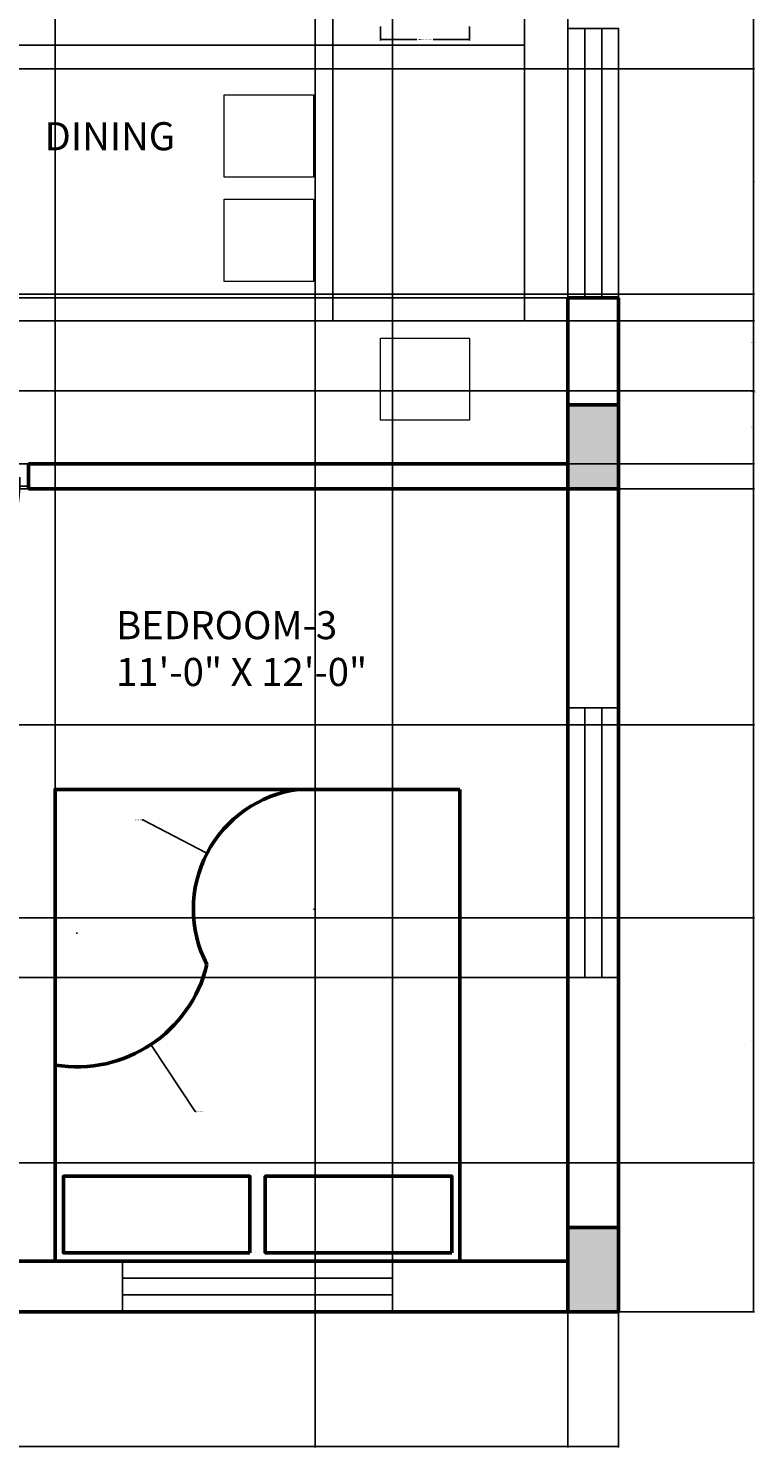
# Model space of a CAD drawing. Units: inches. Extents: x 2480 to 2840, y 795 to 1323.
# Tile 2 of 4: x 2711 to 2840, y 795 to 1047. Entities that reach past the tile are written whole.
import ezdxf

# ---------------------------------------------------------------- set-up
doc = ezdxf.new("R2010")
doc.units = ezdxf.units.IN
for name, color, linetype, lineweight in [('A-ANNO-DIMS', 2, 'Continuous', 18), ('A-AREA-IDEN', 7, 'Continuous', 25), ('COLUMN', 240, 'Continuous', 50), ('door', 140, 'Continuous', 25), ('Furniture', 9, 'Continuous', 18), ('wall', 7, 'Continuous', 50), ('window', 201, 'Continuous', 25)]:
    doc.layers.add(name, color=color, linetype=linetype, lineweight=lineweight)
doc.styles.get("Standard").update_dxf_attribs({"font": 'arial.ttf'})
doc.dimstyles.get("Standard").update_dxf_attribs({"dimtxt": 0.18, "dimasz": 0.18, "dimexe": 0.18, "dimexo": 0.0625, "dimgap": 0.09, "dimtad": 0, "dimtih": 1, "dimtoh": 1, "dimdec": 4, "dimzin": 0, "dimdsep": 46, "dimtxsty": 'Standard', "dimcen": 0.09, "dimadec": 0, "dimazin": 0, "dimtfac": 1, "dimtdec": 4, "dimtofl": 0, "dimtmove": 0, "dimatfit": 3, "dimfxl": 1, "dimtolj": 1, "dimtzin": 0, "dimarcsym": 0})

# ---------------------------------------------------------------- blocks, each defined once
blk = doc.blocks.new('w1')
at = {"layer": 'window'}
for p, q in [((2922.2, 1100.57), (2922.2, 1052.57)), ((2925.2, 1100.57), (2925.2, 1052.57))]:
    blk.add_line(p, q, dxfattribs=at)
blk.add_lwpolyline([(2919.2, 1052.57), (2928.2, 1052.57), (2928.2, 1100.57), (2919.2, 1100.57)], close=True, dxfattribs=at)
blk = doc.blocks.new('d1')
at = {"layer": 'door'}
blk.add_line((3049.73, 1052.02), (3085.73, 1052.02), dxfattribs=at)
blk.add_lwpolyline([(3051.23, 1054.52), (3052.73, 1054.52), (3052.73, 1087.52), (3051.23, 1087.52)], close=True, dxfattribs=at)
for points in [[(3052.73, 1052.02), (3049.73, 1052.02), (3049.73, 1056.02), (3051.23, 1056.02), (3051.23, 1054.52), (3052.73, 1054.52), (3052.73, 1052.02)], [(3082.73, 1052.02), (3085.73, 1052.02), (3085.73, 1056.02), (3084.23, 1056.02), (3084.23, 1054.52), (3082.73, 1054.52), (3082.73, 1052.02)]]:
    blk.add_lwpolyline(points, dxfattribs=at)
blk.add_arc((3051.23, 1054.52), 33.03, 2.6026, 87.3974, dxfattribs=at)
blk = doc.blocks.new('BED')
at = {"layer": 'wall'}
for points in [[(3037.98, 1220.47), (3109.98, 1220.47), (3109.98, 1304.47), (3037.98, 1304.47)], [(3039.4, 1302.95), (3072.6, 1302.95), (3072.6, 1289.33), (3039.4, 1289.33)], [(3075.32, 1302.95), (3108.52, 1302.95), (3108.52, 1289.33), (3075.32, 1289.33)]]:
    blk.add_lwpolyline(points, close=True, dxfattribs=at)
for centre, radius, start, end in [((3106.11, 1246.04), 23.81, 80.6483, 166.366), ((3063.91, 1241.76), 21.48, 277.4854, 27.4236)]:
    blk.add_arc(centre, radius, start, end, dxfattribs=at)
blk = doc.blocks.new('C')
at = {"layer": 'COLUMN'}
h = blk.add_hatch(color=256, dxfattribs=at)
h.dxf.hatch_style = 1
h.paths.add_polyline_path([(3016.24, 1218.72), (3031.24, 1218.72), (3031.24, 1227.72), (3016.24, 1227.72)])
blk.add_lwpolyline([(3016.24, 1218.72), (3031.24, 1218.72), (3031.24, 1227.72), (3016.24, 1227.72)], close=True, dxfattribs=at)
blk = doc.blocks.new('CHAIR-DINING')
blk.add_lwpolyline([(15.88, 0), (0, 0), (0, 14.61), (15.88, 14.61)], close=True)
blk = doc.blocks.new('*D26')
at = {"layer": 'A-ANNO-DIMS', "color": 0, "lineweight": -2, "transparency": 16777216}
for p, q in [((2773.57, 1047.6), (2773.57, 1045.1)), ((2789.45, 1047.6), (2789.45, 1045.1)), ((2773.75, 1045.28), (2780.09, 1045.28)), ((2789.27, 1045.28), (2782.94, 1045.28))]:
    blk.add_line(p, q, dxfattribs=at)
at = {"layer": 'A-ANNO-DIMS', "color": 0, "transparency": 16777216}
for points in [[(2773.75, 1045.31), (2773.75, 1045.25), (2773.57, 1045.28)], [(2789.27, 1045.31), (2789.27, 1045.25), (2789.45, 1045.28)]]:
    blk.add_solid(points, dxfattribs=at)
at = {"layer": 'Defpoints', "color": 0, "transparency": 16777216}
for p in [(2773.57, 1047.66), (2789.45, 1047.66), (2789.45, 1045.28)]:
    blk.add_point(p, dxfattribs=at)
at = {"layer": 'A-ANNO-DIMS', "color": 0, "transparency": 16777216, "insert": (2781.51, 1045.28), "char_height": 0.18, "attachment_point": 5}
blk.add_mtext('\\A1;DINING CHAIR 16 TYP.', dxfattribs=at)
blk = doc.blocks.new('*D28')
at = {"layer": 'A-ANNO-DIMS', "color": 0, "lineweight": -2, "transparency": 16777216}
for p, q in [((2503.95, 836.18), (2503.95, 794.56)), ((2815.95, 818.68), (2815.95, 794.56)), ((2504.13, 794.74), (2659.67, 794.74)), ((2815.77, 794.74), (2660.24, 794.74))]:
    blk.add_line(p, q, dxfattribs=at)
at = {"layer": 'A-ANNO-DIMS', "color": 0, "transparency": 16777216}
for points in [[(2504.13, 794.77), (2504.13, 794.71), (2503.95, 794.74)], [(2815.77, 794.77), (2815.77, 794.71), (2815.95, 794.74)]]:
    blk.add_solid(points, dxfattribs=at)
at = {"layer": 'Defpoints', "color": 0, "transparency": 16777216}
for p in [(2503.95, 836.24), (2815.95, 818.74), (2815.95, 794.74)]:
    blk.add_point(p, dxfattribs=at)
at = {"layer": 'A-ANNO-DIMS', "color": 0, "transparency": 16777216, "insert": (2659.95, 794.74), "char_height": 0.18, "attachment_point": 5}
blk.add_mtext('\\A1;312', dxfattribs=at)
blk = doc.blocks.new('*D29')
at = {"layer": 'A-ANNO-DIMS', "color": 0, "lineweight": -2, "transparency": 16777216}
for p, q in [((2816.02, 1298.74), (2840.14, 1298.74)), ((2839.96, 1298.56), (2839.96, 1058.92)), ((2839.96, 818.92), (2839.96, 1058.56)), ((2816.02, 818.74), (2840.14, 818.74))]:
    blk.add_line(p, q, dxfattribs=at)
at = {"layer": 'A-ANNO-DIMS', "color": 0, "transparency": 16777216}
for points in [[(2839.93, 1298.56), (2839.99, 1298.56), (2839.96, 1298.74)], [(2839.93, 818.92), (2839.99, 818.92), (2839.96, 818.74)]]:
    blk.add_solid(points, dxfattribs=at)
at = {"layer": 'Defpoints', "color": 0, "transparency": 16777216}
for p in [(2815.95, 1298.74), (2839.96, 1298.74), (2815.95, 818.74)]:
    blk.add_point(p, dxfattribs=at)
at = {"layer": 'A-ANNO-DIMS', "color": 0, "transparency": 16777216, "insert": (2839.96, 1058.74), "char_height": 0.18, "attachment_point": 5}
blk.add_mtext('\\A1;480', dxfattribs=at)
blk = doc.blocks.new('*D37')
at = {"layer": 'A-ANNO-DIMS', "color": 0, "lineweight": -2, "transparency": 16777216}
for p, q in [((2806.89, 878.28), (2479.77, 878.28)), ((2479.95, 878.1), (2479.95, 853.19)), ((2479.95, 827.92), (2479.95, 852.83)), ((2806.89, 827.74), (2479.77, 827.74))]:
    blk.add_line(p, q, dxfattribs=at)
at = {"layer": 'A-ANNO-DIMS', "color": 0, "transparency": 16777216}
for points in [[(2479.92, 878.1), (2479.98, 878.1), (2479.95, 878.28)], [(2479.92, 827.92), (2479.98, 827.92), (2479.95, 827.74)]]:
    blk.add_solid(points, dxfattribs=at)
at = {"layer": 'Defpoints', "color": 0, "transparency": 16777216}
for p in [(2479.95, 878.28), (2806.95, 878.28), (2806.95, 827.74)]:
    blk.add_point(p, dxfattribs=at)
at = {"layer": 'A-ANNO-DIMS', "color": 0, "transparency": 16777216, "insert": (2479.95, 853.01), "char_height": 0.18, "attachment_point": 5}
blk.add_mtext('\\A1;50.53', dxfattribs=at)
blk = doc.blocks.new('*D38')
at = {"layer": 'A-ANNO-DIMS', "color": 0, "lineweight": -2, "transparency": 16777216}
for p, q in [((2806.89, 999.24), (2479.77, 999.24)), ((2479.95, 999.06), (2479.95, 984.67)), ((2479.95, 969.92), (2479.95, 984.31)), ((2806.89, 969.74), (2479.77, 969.74))]:
    blk.add_line(p, q, dxfattribs=at)
at = {"layer": 'A-ANNO-DIMS', "color": 0, "transparency": 16777216}
for points in [[(2479.92, 999.06), (2479.98, 999.06), (2479.95, 999.24)], [(2479.92, 969.92), (2479.98, 969.92), (2479.95, 969.74)]]:
    blk.add_solid(points, dxfattribs=at)
at = {"layer": 'Defpoints', "color": 0, "transparency": 16777216}
for p in [(2479.95, 999.24), (2806.95, 999.24), (2806.95, 969.74)]:
    blk.add_point(p, dxfattribs=at)
at = {"layer": 'A-ANNO-DIMS', "color": 0, "transparency": 16777216, "insert": (2479.95, 984.49), "char_height": 0.18, "attachment_point": 5}
blk.add_mtext('\\A1;29.5', dxfattribs=at)
blk = doc.blocks.new('*D41')
at = {"layer": 'A-ANNO-DIMS', "color": 0, "lineweight": -2, "transparency": 16777216}
for p, q in [((2775.71, 827.8), (2775.71, 1322.93)), ((2775.89, 1322.75), (2790.94, 1322.75)), ((2806.77, 1322.75), (2791.73, 1322.75)), ((2806.95, 827.8), (2806.95, 1322.93))]:
    blk.add_line(p, q, dxfattribs=at)
at = {"layer": 'A-ANNO-DIMS', "color": 0, "transparency": 16777216}
for points in [[(2775.89, 1322.78), (2775.89, 1322.72), (2775.71, 1322.75)], [(2806.77, 1322.78), (2806.77, 1322.72), (2806.95, 1322.75)]]:
    blk.add_solid(points, dxfattribs=at)
at = {"layer": 'Defpoints', "color": 0, "transparency": 16777216}
for p in [(2806.95, 1322.75), (2775.71, 827.74), (2806.95, 827.74)]:
    blk.add_point(p, dxfattribs=at)
at = {"layer": 'A-ANNO-DIMS', "color": 0, "transparency": 16777216, "insert": (2791.33, 1322.75), "char_height": 0.18, "attachment_point": 5}
blk.add_mtext('\\A1;31.24', dxfattribs=at)
blk = doc.blocks.new('*D46')
at = {"layer": 'A-ANNO-DIMS', "color": 0, "lineweight": -2, "transparency": 16777216}
for p, q in [((2610.02, 888.87), (2840.14, 888.87)), ((2839.96, 888.69), (2839.96, 867.24)), ((2839.96, 845.42), (2839.96, 866.87)), ((2610.02, 845.24), (2840.14, 845.24))]:
    blk.add_line(p, q, dxfattribs=at)
at = {"layer": 'A-ANNO-DIMS', "color": 0, "transparency": 16777216}
for points in [[(2839.93, 888.69), (2839.99, 888.69), (2839.96, 888.87)], [(2839.93, 845.42), (2839.99, 845.42), (2839.96, 845.24)]]:
    blk.add_solid(points, dxfattribs=at)
at = {"layer": 'Defpoints', "color": 0, "transparency": 16777216}
for p in [(2609.95, 888.87), (2839.96, 888.87), (2609.95, 845.24)]:
    blk.add_point(p, dxfattribs=at)
at = {"layer": 'A-ANNO-DIMS', "color": 0, "transparency": 16777216, "insert": (2839.96, 867.06), "char_height": 0.18, "attachment_point": 5}
blk.add_mtext('\\A1;43.63', dxfattribs=at)
blk = doc.blocks.new('*D49')
at = {"layer": 'A-ANNO-DIMS', "color": 0, "lineweight": -2, "transparency": 16777216}
for p, q in [((2610.02, 965.24), (2840.14, 965.24)), ((2839.96, 965.06), (2839.96, 944.42)), ((2839.96, 923.42), (2839.96, 944.06)), ((2610.02, 923.24), (2840.14, 923.24))]:
    blk.add_line(p, q, dxfattribs=at)
at = {"layer": 'A-ANNO-DIMS', "color": 0, "transparency": 16777216}
for points in [[(2839.93, 965.06), (2839.99, 965.06), (2839.96, 965.24)], [(2839.93, 923.42), (2839.99, 923.42), (2839.96, 923.24)]]:
    blk.add_solid(points, dxfattribs=at)
at = {"layer": 'Defpoints', "color": 0, "transparency": 16777216}
for p in [(2609.95, 965.24), (2839.96, 965.24), (2609.95, 923.24)]:
    blk.add_point(p, dxfattribs=at)
at = {"layer": 'A-ANNO-DIMS', "color": 0, "transparency": 16777216, "insert": (2839.96, 944.24), "char_height": 0.18, "attachment_point": 5}
blk.add_mtext('\\A1;42', dxfattribs=at)
blk = doc.blocks.new('*D51')
at = {"layer": 'A-ANNO-DIMS', "color": 0, "lineweight": -2, "transparency": 16777216}
for p, q in [((2761.95, 1289.68), (2761.95, 794.56)), ((2806.95, 1289.68), (2806.95, 794.56)), ((2762.13, 794.74), (2784.23, 794.74)), ((2806.77, 794.74), (2784.68, 794.74))]:
    blk.add_line(p, q, dxfattribs=at)
at = {"layer": 'A-ANNO-DIMS', "color": 0, "transparency": 16777216}
for points in [[(2762.13, 794.77), (2762.13, 794.71), (2761.95, 794.74)], [(2806.77, 794.77), (2806.77, 794.71), (2806.95, 794.74)]]:
    blk.add_solid(points, dxfattribs=at)
at = {"layer": 'Defpoints', "color": 0, "transparency": 16777216}
for p in [(2761.95, 1289.74), (2806.95, 1289.74), (2806.95, 794.74)]:
    blk.add_point(p, dxfattribs=at)
at = {"layer": 'A-ANNO-DIMS', "color": 0, "transparency": 16777216, "insert": (2784.45, 794.74), "char_height": 0.18, "attachment_point": 5}
blk.add_mtext('\\A1;45', dxfattribs=at)
blk = doc.blocks.new('*D53')
at = {"layer": 'A-ANNO-DIMS', "color": 0, "lineweight": -2, "transparency": 16777216}
for p, q in [((2565.4, 1040.02), (2840.14, 1040.02)), ((2839.96, 1039.84), (2839.96, 1020.15)), ((2839.96, 1000.1), (2839.96, 1019.79)), ((2565.4, 999.92), (2840.14, 999.92))]:
    blk.add_line(p, q, dxfattribs=at)
at = {"layer": 'A-ANNO-DIMS', "color": 0, "transparency": 16777216}
for points in [[(2839.93, 1039.84), (2839.99, 1039.84), (2839.96, 1040.02)], [(2839.93, 1000.1), (2839.99, 1000.1), (2839.96, 999.92)]]:
    blk.add_solid(points, dxfattribs=at)
at = {"layer": 'Defpoints', "color": 0, "transparency": 16777216}
for p in [(2565.34, 1040.02), (2839.96, 1040.02), (2565.34, 999.92)]:
    blk.add_point(p, dxfattribs=at)
at = {"layer": 'A-ANNO-DIMS', "color": 0, "transparency": 16777216, "insert": (2839.96, 1019.97), "char_height": 0.18, "attachment_point": 5}
blk.add_mtext('\\A1;40.1', dxfattribs=at)
blk = doc.blocks.new('*D57')
at = {"layer": 'A-ANNO-DIMS', "color": 0, "lineweight": -2, "transparency": 16777216}
for p, q in [((2765.09, 995.24), (2765.09, 1322.93)), ((2765.27, 1322.75), (2781.68, 1322.75)), ((2799.02, 1322.75), (2782.61, 1322.75)), ((2799.2, 995.24), (2799.2, 1322.93))]:
    blk.add_line(p, q, dxfattribs=at)
at = {"layer": 'A-ANNO-DIMS', "color": 0, "transparency": 16777216}
for points in [[(2765.27, 1322.78), (2765.27, 1322.72), (2765.09, 1322.75)], [(2799.02, 1322.78), (2799.02, 1322.72), (2799.2, 1322.75)]]:
    blk.add_solid(points, dxfattribs=at)
at = {"layer": 'Defpoints', "color": 0, "transparency": 16777216}
for p in [(2799.2, 1322.75), (2765.09, 995.18), (2799.2, 995.18)]:
    blk.add_point(p, dxfattribs=at)
at = {"layer": 'A-ANNO-DIMS', "color": 0, "transparency": 16777216, "insert": (2782.14, 1322.75), "char_height": 0.18, "attachment_point": 5}
blk.add_mtext('\\A1;34.114', dxfattribs=at)
blk = doc.blocks.new('*D58')
at = {"layer": 'A-ANNO-DIMS', "color": 0, "lineweight": -2, "transparency": 16777216}
for p, q in [((2799.14, 1044.23), (2479.77, 1044.23)), ((2479.95, 1044.05), (2479.95, 1019.89)), ((2479.95, 995.36), (2479.95, 1019.52)), ((2799.14, 995.18), (2479.77, 995.18))]:
    blk.add_line(p, q, dxfattribs=at)
at = {"layer": 'A-ANNO-DIMS', "color": 0, "transparency": 16777216}
for points in [[(2479.92, 1044.05), (2479.98, 1044.05), (2479.95, 1044.23)], [(2479.92, 995.36), (2479.98, 995.36), (2479.95, 995.18)]]:
    blk.add_solid(points, dxfattribs=at)
at = {"layer": 'Defpoints', "color": 0, "transparency": 16777216}
for p in [(2479.95, 1044.23), (2799.2, 1044.23), (2799.2, 995.18)]:
    blk.add_point(p, dxfattribs=at)
at = {"layer": 'A-ANNO-DIMS', "color": 0, "transparency": 16777216, "insert": (2479.95, 1019.7), "char_height": 0.18, "attachment_point": 5}
blk.add_mtext('\\A1;49.06', dxfattribs=at)
blk = doc.blocks.new('*D60')
at = {"layer": 'A-ANNO-DIMS', "color": 0, "lineweight": -2, "transparency": 16777216}
for p, q in [((2519.7, 982.73), (2840.14, 982.73)), ((2839.96, 982.55), (2839.96, 976.42)), ((2839.96, 969.92), (2839.96, 976.05)), ((2513.02, 969.74), (2840.14, 969.74))]:
    blk.add_line(p, q, dxfattribs=at)
at = {"layer": 'A-ANNO-DIMS', "color": 0, "transparency": 16777216}
for points in [[(2839.93, 982.55), (2839.99, 982.55), (2839.96, 982.73)], [(2839.93, 969.92), (2839.99, 969.92), (2839.96, 969.74)]]:
    blk.add_solid(points, dxfattribs=at)
at = {"layer": 'Defpoints', "color": 0, "transparency": 16777216}
for p in [(2519.64, 982.73), (2839.96, 982.73), (2512.95, 969.74)]:
    blk.add_point(p, dxfattribs=at)
at = {"layer": 'A-ANNO-DIMS', "color": 0, "transparency": 16777216, "insert": (2839.96, 976.23), "char_height": 0.18, "attachment_point": 5}
blk.add_mtext('\\A1;12.984', dxfattribs=at)
blk = doc.blocks.new('*D61')
at = {"layer": 'A-ANNO-DIMS', "color": 0, "lineweight": -2, "transparency": 16777216}
for p, q in [((2799.2, 1044.3), (2799.2, 1322.93)), ((2799.38, 1322.75), (2802.69, 1322.75)), ((2806.77, 1322.75), (2803.47, 1322.75)), ((2806.95, 1047.3), (2806.95, 1322.93))]:
    blk.add_line(p, q, dxfattribs=at)
at = {"layer": 'A-ANNO-DIMS', "color": 0, "transparency": 16777216}
for points in [[(2799.38, 1322.78), (2799.38, 1322.72), (2799.2, 1322.75)], [(2806.77, 1322.78), (2806.77, 1322.72), (2806.95, 1322.75)]]:
    blk.add_solid(points, dxfattribs=at)
at = {"layer": 'Defpoints', "color": 0, "transparency": 16777216}
for p in [(2799.2, 1322.75), (2806.95, 1047.24), (2799.2, 1044.23)]:
    blk.add_point(p, dxfattribs=at)
at = {"layer": 'A-ANNO-DIMS', "color": 0, "transparency": 16777216, "insert": (2803.08, 1322.75), "char_height": 0.18, "attachment_point": 5}
blk.add_mtext('\\A1;7.752', dxfattribs=at)
blk = doc.blocks.new('*D62')
at = {"layer": 'A-ANNO-DIMS', "color": 0, "lineweight": -2, "transparency": 16777216}
for p, q in [((2799.26, 995.18), (2840.14, 995.18)), ((2839.96, 995), (2839.96, 982.64)), ((2839.96, 969.92), (2839.96, 982.28)), ((2807.02, 969.74), (2840.14, 969.74))]:
    blk.add_line(p, q, dxfattribs=at)
at = {"layer": 'A-ANNO-DIMS', "color": 0, "transparency": 16777216}
for points in [[(2839.93, 995), (2839.99, 995), (2839.96, 995.18)], [(2839.93, 969.92), (2839.99, 969.92), (2839.96, 969.74)]]:
    blk.add_solid(points, dxfattribs=at)
at = {"layer": 'Defpoints', "color": 0, "transparency": 16777216}
for p in [(2799.2, 995.18), (2839.96, 995.18), (2806.95, 969.74)]:
    blk.add_point(p, dxfattribs=at)
at = {"layer": 'A-ANNO-DIMS', "color": 0, "transparency": 16777216, "insert": (2839.96, 982.46), "char_height": 0.18, "attachment_point": 5}
blk.add_mtext('\\A1;25.436', dxfattribs=at)
blk = doc.blocks.new('*D64')
at = {"layer": 'A-ANNO-DIMS', "color": 0, "lineweight": -2, "transparency": 16777216}
for p, q in [((2550, 999.92), (2840.14, 999.92)), ((2839.96, 999.74), (2839.96, 991.5)), ((2839.96, 982.91), (2839.96, 991.14)), ((2544.07, 982.73), (2840.14, 982.73))]:
    blk.add_line(p, q, dxfattribs=at)
at = {"layer": 'A-ANNO-DIMS', "color": 0, "transparency": 16777216}
for points in [[(2839.93, 999.74), (2839.99, 999.74), (2839.96, 999.92)], [(2839.93, 982.91), (2839.99, 982.91), (2839.96, 982.73)]]:
    blk.add_solid(points, dxfattribs=at)
at = {"layer": 'Defpoints', "color": 0, "transparency": 16777216}
for p in [(2549.93, 999.92), (2839.96, 999.92), (2544, 982.73)]:
    blk.add_point(p, dxfattribs=at)
at = {"layer": 'A-ANNO-DIMS', "color": 0, "transparency": 16777216, "insert": (2839.96, 991.32), "char_height": 0.18, "attachment_point": 5}
blk.add_mtext('\\A1;17.193', dxfattribs=at)
blk = doc.blocks.new('*D67')
at = {"layer": 'A-ANNO-DIMS', "color": 0, "lineweight": -2, "transparency": 16777216}
for p, q in [((2674.95, 827.8), (2674.95, 1322.93)), ((2675.13, 1322.75), (2694.94, 1322.75)), ((2715.53, 1322.75), (2695.73, 1322.75)), ((2715.71, 827.8), (2715.71, 1322.93))]:
    blk.add_line(p, q, dxfattribs=at)
at = {"layer": 'A-ANNO-DIMS', "color": 0, "transparency": 16777216}
for points in [[(2675.13, 1322.78), (2675.13, 1322.72), (2674.95, 1322.75)], [(2715.53, 1322.78), (2715.53, 1322.72), (2715.71, 1322.75)]]:
    blk.add_solid(points, dxfattribs=at)
at = {"layer": 'Defpoints', "color": 0, "transparency": 16777216}
for p in [(2715.71, 1322.75), (2674.95, 827.74), (2715.71, 827.74)]:
    blk.add_point(p, dxfattribs=at)
at = {"layer": 'A-ANNO-DIMS', "color": 0, "transparency": 16777216, "insert": (2695.33, 1322.75), "char_height": 0.18, "attachment_point": 5}
blk.add_mtext('\\A1;40.76', dxfattribs=at)
blk = doc.blocks.new('*D72')
at = {"layer": 'A-ANNO-DIMS', "color": 0, "lineweight": -2, "transparency": 16777216}
for p, q in [((2731.14, 906.34), (2731.32, 906.34)), ((2731.32, 906.34), (2742.58, 900.46)), ((2761.7, 890.44), (2761.88, 890.44)), ((2761.79, 890.35), (2761.79, 890.53))]:
    blk.add_line(p, q, dxfattribs=at)
at = {"layer": 'A-ANNO-DIMS', "color": 0, "transparency": 16777216}
blk.add_solid([(2742.6, 900.49), (2742.57, 900.43), (2742.74, 900.38)], dxfattribs=at)
at = {"layer": 'Defpoints', "color": 0, "transparency": 16777216}
for p in [(2742.74, 900.38), (2761.79, 890.44)]:
    blk.add_point(p, dxfattribs=at)
at = {"layer": 'A-ANNO-DIMS', "color": 0, "transparency": 16777216, "insert": (2730.46, 906.34), "char_height": 0.18, "attachment_point": 5}
blk.add_mtext('\\A1;3X R21.48', dxfattribs=at)
blk = doc.blocks.new('*D73')
at = {"layer": 'A-ANNO-DIMS', "color": 0, "lineweight": -2, "transparency": 16777216}
for p, q in [((2719.49, 886.16), (2719.67, 886.16)), ((2719.58, 886.07), (2719.58, 886.25)), ((2740.61, 854.4), (2732.83, 866.16)), ((2740.79, 854.4), (2740.61, 854.4))]:
    blk.add_line(p, q, dxfattribs=at)
at = {"layer": 'A-ANNO-DIMS', "color": 0, "transparency": 16777216}
blk.add_solid([(2732.85, 866.18), (2732.8, 866.15), (2732.73, 866.31)], dxfattribs=at)
at = {"layer": 'Defpoints', "color": 0, "transparency": 16777216}
for p in [(2719.58, 886.16), (2732.73, 866.31)]:
    blk.add_point(p, dxfattribs=at)
at = {"layer": 'A-ANNO-DIMS', "color": 0, "transparency": 16777216, "insert": (2741.45, 854.4), "char_height": 0.18, "attachment_point": 5}
blk.add_mtext('\\A1;3X R23.81', dxfattribs=at)

msp = doc.modelspace()

# ---------------------------------------------------------------- linework, layer by layer
at = {"layer": 'Furniture'}
msp.add_lwpolyline([(2765.0875, 1044.2327), (2799.2019, 1044.2327), (2799.2019, 995.1772), (2765.0875, 995.1772)], close=True, dxfattribs=at)
at = {"layer": 'wall'}
for p, q in [((2806.9535, 969.7416), (2806.9535, 999.2416)), ((2806.9535, 999.2416), (2815.9535, 999.2416)), ((2815.9535, 818.7416), (2815.9535, 999.2416)), ((2806.9535, 969.7416), (2710.9535, 969.7416)), ((2710.9535, 965.2416), (2710.9535, 969.7416)), ((2806.9535, 965.2416), (2710.9535, 965.2416)), ((2806.9535, 827.7416), (2806.9535, 965.2416)), ((2674.9535, 827.7416), (2806.9535, 827.7416)), ((2670.4535, 818.7416), (2815.9535, 818.7416))]:
    msp.add_line(p, q, dxfattribs=at)

# ---------------------------------------------------------------- block references
at = {"layer": 'COLUMN', "rotation": 270}
for p in [(1588.2303, 3996.4817), (1588.2303, 3849.9817)]:
    msp.add_blockref('C', p, dxfattribs=at)
at = {"layer": 'door', "xscale": -1, "rotation": 180}
msp.add_blockref('d1', (-374.7789, 2021.7615), dxfattribs=at)
at = {"layer": 'Furniture'}
for p in [(2745.7756, 1020.7777), (2745.7756, 1002.2015), (2773.571, 977.4934)]:
    msp.add_blockref('CHAIR-DINING', p, dxfattribs=at)
at = {"layer": 'Furniture', "rotation": 180}
msp.add_blockref('BED', (5825.6933, 2132.2076), dxfattribs=at)
at = {"layer": 'window'}
for p in [(-112.2506, -53.327), (-112.2506, -174.2933)]:
    msp.add_blockref('w1', p, dxfattribs=at)
at = {"layer": 'window', "rotation": 90}
msp.add_blockref('w1', (3828.2834, -2100.4626), dxfattribs=at)

# ---------------------------------------------------------------- texts
at = {"layer": 'A-AREA-IDEN', "char_height": 5, "attachment_point": 1}
for s, insert in [('DINING', (2713.8122, 1030.5385)), ('BEDROOM-3\\P11\'-0" X 12\'-0"', (2726.5525, 943.4891))]:
    msp.add_mtext_dynamic_manual_height_columns(s, width=47.7919, gutter_width=12.5, heights=[0], dxfattribs=dict(at, insert=insert))

# ---------------------------------------------------------------- dimensions: what is measured, and where the dimension line sits
at = {"layer": 'A-ANNO-DIMS'}
for base, p1, p2, override, picture, middle in [((2715.7148, 1322.7466), (2674.9535, 827.7416), (2715.7148, 827.7416), {"dimdec": 2, "dimlfac": 1, "dimrnd": 0, "dimzin": 0, "dimdsep": 46, "dimlunit": 2}, '*D67', (2695.3342, 1322.7466)), ((2799.2019, 1322.7466), (2765.0875, 995.1772), (2799.2019, 995.1772), {"dimdec": 3, "dimlfac": 1, "dimrnd": 0, "dimzin": 0, "dimdsep": 46, "dimlunit": 2}, '*D57', (2782.1447, 1322.7466)), ((2806.9535, 1322.7466), (2775.7148, 827.7416), (2806.9535, 827.7416), {"dimdec": 2, "dimlfac": 1, "dimrnd": 0, "dimzin": 0, "dimdsep": 46, "dimlunit": 2}, '*D41', (2791.3342, 1322.7466)), ((2799.2019, 1322.7466), (2806.9535, 1047.2416), (2799.2019, 1044.2327), {"dimdec": 3, "dimlfac": 1, "dimrnd": 0, "dimzin": 0, "dimdsep": 46, "dimlunit": 2}, '*D61', (2803.0777, 1322.7466)), ((2806.9535, 794.7366), (2761.9535, 1289.7416), (2806.9535, 1289.7416), {"dimdec": 0, "dimlfac": 1, "dimrnd": 0, "dimzin": 0, "dimdsep": 46, "dimlunit": 2}, '*D51', (2784.4535, 794.7366)), ((2815.9535, 794.7366), (2503.9535, 836.2416), (2815.9535, 818.7416), {"dimdec": 0, "dimlfac": 1, "dimrnd": 0, "dimzin": 0, "dimdsep": 46, "dimlunit": 2}, '*D28', (2659.9535, 794.7366))]:
    dim = msp.add_linear_dim(base=base, p1=p1, p2=p2, dimstyle='Standard', override=override, dxfattribs=at)
    dim.commit()
    dim.dimension.update_dxf_attribs({"geometry": picture, "text_midpoint": middle})
for base, p1, p2, override, picture, middle in [((2839.9585, 1298.7416), (2815.9535, 818.7416), (2815.9535, 1298.7416), {"dimdec": 0, "dimlfac": 1, "dimrnd": 0, "dimzin": 0, "dimdsep": 46, "dimlunit": 2}, '*D29', (2839.9585, 1058.7416)), ((2479.9485, 1044.2327), (2799.2019, 995.1772), (2799.2019, 1044.2327), {"dimdec": 2, "dimlfac": 1, "dimrnd": 0, "dimzin": 0, "dimdsep": 46, "dimlunit": 2}, '*D58', (2479.9485, 1019.705)), ((2839.9585, 1040.0192), (2565.3407, 999.9194), (2565.3407, 1040.0192), {"dimdec": 1, "dimlfac": 1, "dimrnd": 0, "dimzin": 0, "dimdsep": 46, "dimlunit": 2}, '*D53', (2839.9585, 1019.9693)), ((2479.9485, 999.2416), (2806.9535, 969.7416), (2806.9535, 999.2416), {"dimdec": 1, "dimlfac": 1, "dimrnd": 0, "dimzin": 0, "dimdsep": 46, "dimlunit": 2}, '*D38', (2479.9485, 984.4916)), ((2839.9585, 999.9194), (2544.0036, 982.726), (2549.9325, 999.9194), {"dimdec": 3, "dimlfac": 1, "dimrnd": 0, "dimzin": 0, "dimdsep": 46, "dimlunit": 2}, '*D64', (2839.9585, 991.3227)), ((2839.9585, 995.1772), (2806.9535, 969.7416), (2799.2019, 995.1772), {"dimdec": 3, "dimlfac": 1, "dimrnd": 0, "dimzin": 0, "dimdsep": 46, "dimlunit": 2}, '*D62', (2839.9585, 982.4594)), ((2839.9585, 982.726), (2512.9535, 969.7416), (2519.6396, 982.726), {"dimdec": 3, "dimlfac": 1, "dimrnd": 0, "dimzin": 0, "dimdsep": 46, "dimlunit": 2}, '*D60', (2839.9585, 976.2338)), ((2839.9585, 965.2416), (2609.9535, 923.2416), (2609.9535, 965.2416), {"dimdec": 0, "dimlfac": 1, "dimrnd": 0, "dimzin": 0, "dimdsep": 46, "dimlunit": 2}, '*D49', (2839.9585, 944.2416)), ((2839.9585, 888.8711), (2609.9535, 845.2416), (2609.9535, 888.8711), {"dimdec": 2, "dimlfac": 1, "dimrnd": 0, "dimzin": 0, "dimdsep": 46, "dimlunit": 2}, '*D46', (2839.9585, 867.0564)), ((2479.9485, 878.2753), (2806.9535, 827.7416), (2806.9535, 878.2753), {"dimdec": 2, "dimlfac": 1, "dimrnd": 0, "dimzin": 0, "dimdsep": 46, "dimlunit": 2}, '*D37', (2479.9485, 853.0085))]:
    dim = msp.add_linear_dim(base=base, p1=p1, p2=p2, angle=90, dimstyle='Standard', override=override, dxfattribs=at)
    dim.commit()
    dim.dimension.update_dxf_attribs({"geometry": picture, "text_midpoint": middle})
dim = msp.add_linear_dim(base=(2789.4549, 1045.2768), p1=(2773.571, 1047.6594), p2=(2789.4549, 1047.6594), text='DINING CHAIR <> TYP.', dimstyle='Standard', override={"dimdec": 0, "dimlfac": 1, "dimrnd": 0, "dimzin": 0, "dimdsep": 46, "dimlunit": 2}, dxfattribs=at)
dim.commit()
dim.dimension.update_dxf_attribs({"geometry": '*D26', "text_midpoint": (2781.513, 1045.2768)})
for center, mpoint, picture, middle in [((2761.7876, 890.4445), (2742.7423, 900.3779), '*D72', (2730.4617, 906.3378)), ((2719.5835, 886.1637), (2732.7271, 866.3118), '*D73', (2741.4491, 854.4006))]:
    dim = msp.add_radius_dim(center=center, mpoint=mpoint, text='3X <>', dimstyle='Standard', override={"dimdec": 2, "dimlfac": 1, "dimrnd": 0, "dimzin": 0, "dimdsep": 46, "dimlunit": 2}, dxfattribs=at)
    dim.commit()
    dim.dimension.update_dxf_attribs({"geometry": picture, "text_midpoint": middle, "dimtype": 164})

doc.saveas('drawing.dxf')
